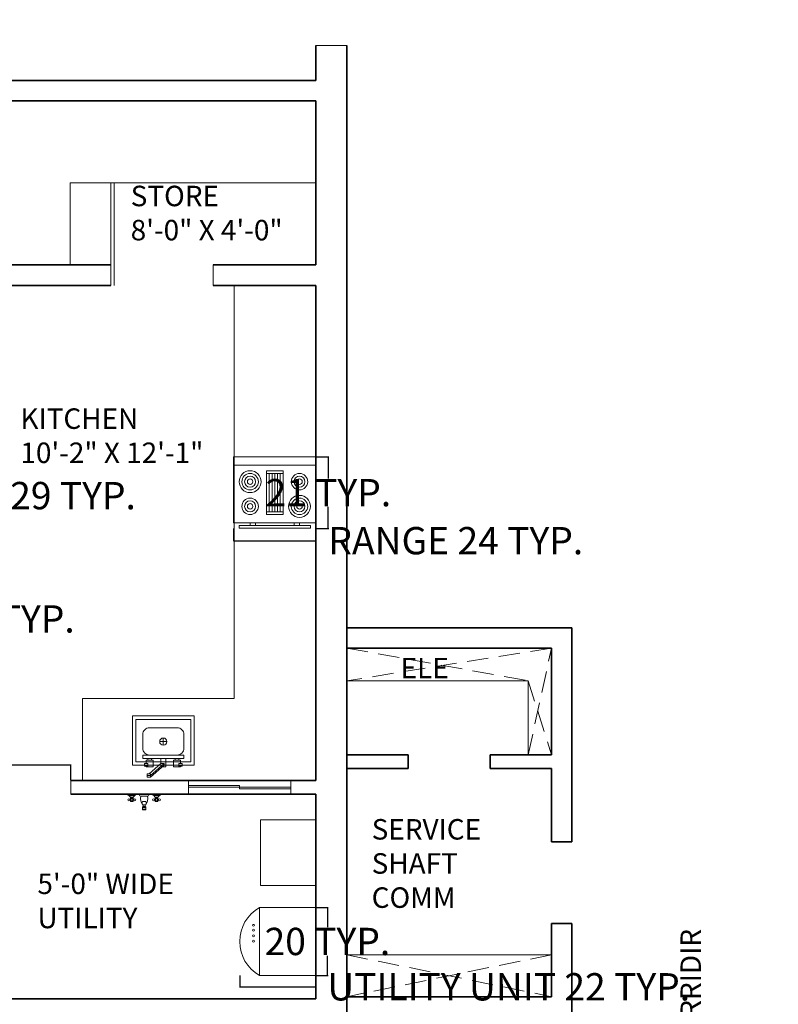
# Model space of a CAD drawing. Units: inches. Extents: x 3343 to 4790, y 1140 to 2641.
# Tile 5 of 10: x 3881 to 4104, y 2022 to 2310. Entities that reach past the tile are written whole.
import ezdxf

# ---------------------------------------------------------------- set-up
doc = ezdxf.new("R2010")
doc.units = ezdxf.units.IN
doc.header["$LTSCALE"] = 5
doc.header["$MEASUREMENT"] = 0
doc.linetypes.add('HIDDEN', pattern=[0.375, 0.25, -0.125])
for name, color, linetype, lineweight in [('A-ANNO-DIMS', 2, 'Continuous', 18), ('A-AREA-IDEN', 7, 'Continuous', 18), ('A-DOOR', 3, 'Continuous', 18), ('A-EQPM', 9, 'Continuous', 18), ('A-FLOR-CASE', 9, 'Continuous', 18), ('A-FLOR-FIXT', 9, 'Continuous', 18), ('A-FLOR-HIDN', 8, 'HIDDEN', 13), ('A-FLOR-SHFT', 8, 'Continuous', 18), ('A-GLAZ', 4, 'Continuous', 18), ('A-WALL', 7, 'Continuous', 35)]:
    doc.layers.add(name, color=color, linetype=linetype, lineweight=lineweight)
doc.styles.get("Standard").update_dxf_attribs({"font": 'arial.ttf'})
doc.dimstyles.get("Standard").update_dxf_attribs({"dimtxt": 8, "dimasz": 0.18, "dimexe": 0.18, "dimexo": 0.0625, "dimgap": 0.09, "dimtad": 0, "dimtih": 1, "dimtoh": 1, "dimdec": 1, "dimzin": 0, "dimdsep": 46, "dimlunit": 3, "dimtxsty": 'Standard', "dimcen": 0.09, "dimadec": 0, "dimazin": 0, "dimtfac": 1, "dimtdec": 1, "dimtofl": 0, "dimtmove": 0, "dimatfit": 3, "dimfxl": 1, "dimtolj": 1, "dimtzin": 0, "dimarcsym": 0})

# ---------------------------------------------------------------- blocks, each defined once
blk = doc.blocks.new('Faucet - Bathroom front')
for p, q in [((-0.5, 4.25), (0.5, 4.25)), ((0.5, 3.75), (-0.5, 3.75)), ((-0.5, 3), (0.5, 3)), ((-0.25, 3), (-0.25, 3.5)), ((0.25, 3.5), (0.25, 3)), ((-5, 0), (-2.25, 0)), ((-4.5087, 0.25), (-2.7408, 0.25)), ((-4, 1.625), (-4.25, 1.625)), ((-4, 1.375), (-4.25, 1.375)), ((-3.1442, 0.75), (-4.0979, 0.75)), ((-3.25, 1.625), (-3, 1.625)), ((-3.25, 1.375), (-3, 1.375)), ((-1.5, 0), (1.5, 0)), ((-1, 0.5), (1, 0.5)), ((0.5, 2), (-0.5, 2)), ((2.25, 0), (5, 0)), ((2.7413, 0.25), (4.5092, 0.25)), ((3.25, 1.625), (3, 1.625)), ((3.25, 1.375), (3, 1.375)), ((4.1058, 0.75), (3.1521, 0.75)), ((4, 1.625), (4.25, 1.625)), ((4, 1.375), (4.25, 1.375))]:
    blk.add_line(p, q)
for points in [[(-0.5, 3.75), (-0.5, 4.25)], [(-0.25, 4.5), (0.25, 4.5)], [(0.25, 3.5), (-0.25, 3.5)], [(0.5, 4.25), (0.5, 3.75)]]:
    blk.add_lwpolyline(points)
for points in [[(-4, 1), (-4, 2), (-3.25, 2), (-3.25, 1)], [(3.25, 1), (3.25, 2), (4, 2), (4, 1)]]:
    blk.add_lwpolyline(points, close=True)
for centre in [(-4.5, 1.5), (-3.625, 1.5), (-2.75, 1.5), (2.75, 1.5), (3.625, 1.5), (4.5, 1.5)]:
    blk.add_circle(centre, 0.2795)
for centre, radius, start, end in [((3, 1), 4.0311, 150.2551, 187.125), ((0.6413, 2.5), 1.246, 156.3417, 203.6583), ((-0.2575, 4.2575), 0.2426, 88.22243, 181.7776), ((-0.2575, 3.7425), 0.2426, 178.2224, 271.7776), ((0.2575, 4.2575), 0.2426, 358.2224, 91.77757), ((0.2575, 3.7425), 0.2426, 268.2224, 1.777565), ((-3, 1), 4.0311, 352.875, 29.74488), ((-0.6413, 2.5), 1.246, 336.3417, 23.65835), ((-5.375, 1.375), 1.4252, 285.2551, 344.7449), ((-1.875, 1.375), 1.4252, 195.2551, 254.7449), ((-0.7962, -0.2038), 0.7327, 106.1502, 163.8498), ((0.7962, -0.2038), 0.7327, 16.1502, 73.84979), ((1.875, 1.375), 1.4252, 285.2551, 344.7449), ((5.375, 1.375), 1.4252, 195.2551, 254.7449)]:
    blk.add_arc(centre, radius, start, end)
blk = doc.blocks.new('Range-Oven - 30 in top')
for p, q in [((0, -3), (30, -3)), ((12, -6), (18, -6)), ((13, -20), (13, -6)), ((14, -6), (14, -20)), ((15, -20), (15, -6)), ((16, -6), (16, -20)), ((17, -20), (17, -6)), ((18, -20), (12, -20)), ((6, -24), (6, -25)), ((8, -25), (8, -24)), ((22, -25), (22, -24)), ((24, -24), (24, -25))]:
    blk.add_line(p, q)
for points in [[(0, -24), (0, 0), (30, 0), (30, -24)], [(12, -21), (12, -5), (18, -5), (18, -21)], [(2, -26), (2, -25), (28, -25), (28, -26)]]:
    blk.add_lwpolyline(points, close=True)
for centre, radius in [((6, -9), 4), ((6, -9), 3), ((6, -9), 2), ((24, -9), 3), ((24, -9), 2), ((6, -9), 1), ((24, -9), 1), ((24, -18), 4), ((6, -18), 3), ((6, -18), 2), ((6, -18), 1), ((24, -18), 3), ((24, -18), 2), ((24, -18), 1)]:
    blk.add_circle(centre, radius)
blk = doc.blocks.new('Faucet - kit sink front')
for p, q in [((-0.25, 3), (3.75, 6.5)), ((3.75, 6), (-0.25, 2.5)), ((3.75, 6), (3.75, 6.5)), ((3.75, 6.5), (4.75, 6.5)), ((3.75, 5.5), (3.75, 6)), ((4.75, 6), (3.75, 6)), ((4.75, 6.5), (4.75, 6)), ((4.75, 6), (4.75, 5.5)), ((-0.75, 3.5), (0.3192, 3.5)), ((-0.75, 1), (-0.75, 3.5)), ((-0.25, 2.5), (-0.25, 3)), ((4.1921, 5.5041), (0.75, 2.5)), ((4.75, 5.5), (3.75, 5.5)), ((-4.5, 1), (-4.5, 1.5)), ((-3.5, 1.5), (-3.5, 1)), ((0.75, 2.5), (-0.25, 2.5)), ((0.75, 2.5), (0.75, 1)), ((3.5, 1.5), (3.5, 1)), ((4.5, 1), (4.5, 1.5))]:
    blk.add_line(p, q)
for points in [[(-5.5, 2.5), (-5.5, 3.25), (-4.5, 3.25), (-4.5, 2.5)], [(5.5, 2.5), (5.5, 3.25), (4.5, 3.25), (4.5, 2.5)], [(-6, 0), (-6, 1), (6, 1), (6, 0)]]:
    blk.add_lwpolyline(points, close=True)
for points in [[(-5, 3.2513), (-5, 3.5), (-3, 3.5), (-3, 1.5), (-5, 1.5), (-5, 2.5)], [(5, 3.2513), (5, 3.5), (3, 3.5), (3, 1.5), (5, 1.5), (5, 2.5)]]:
    blk.add_lwpolyline(points)
blk = doc.blocks.new('UTILITY-APPLIANCE')
blk.add_lwpolyline([(22.35, 19.84), (5.78, 19.84), (5.78, 0), (22.35, 0)], close=True)
for centre in [(4.05, 14.66), (4.05, 13.23), (4.05, 11.58), (4.05, 10.02)]:
    blk.add_circle(centre, 0.275)
blk.add_arc((11.41, 9.92), 11.41, 119.598, 240.402)
blk = doc.blocks.new('DOOR-30IN-4IN-JAMB-DBL-LINE')
at = {"ltscale": 5}
for p, q in [((29, 0), (29, 30)), ((30, 0), (30, 30)), ((0, 4), (0, 0)), ((30, 4), (30, 0))]:
    blk.add_line(p, q, dxfattribs=at)
blk = doc.blocks.new('*D51')
at = {"layer": 'A-ANNO-DIMS', "color": 0, "lineweight": -2, "ltscale": 5, "transparency": 16777216}
for p, q in [((3806.15, 2137.1), (3806.15, 2134.27)), ((3824.22, 2137.1), (3824.22, 2134.27)), ((3806.33, 2134.45), (3824.04, 2134.45)), ((3824.22, 2134.45), (3824.4, 2134.45))]:
    blk.add_line(p, q, dxfattribs=at)
at = {"layer": 'A-ANNO-DIMS', "color": 0, "ltscale": 5, "transparency": 16777216}
for points in [[(3806.33, 2134.48), (3806.33, 2134.42), (3806.15, 2134.45)], [(3824.04, 2134.48), (3824.04, 2134.42), (3824.22, 2134.45)]]:
    blk.add_solid(points, dxfattribs=at)
at = {"layer": 'Defpoints', "color": 0, "ltscale": 5, "transparency": 16777216}
for p in [(3806.15, 2137.16), (3824.22, 2137.16), (3824.22, 2134.45)]:
    blk.add_point(p, dxfattribs=at)
at = {"layer": 'A-ANNO-DIMS', "color": 0, "ltscale": 5, "transparency": 16777216, "insert": (3862.1, 2134.45), "char_height": 8, "attachment_point": 5}
blk.add_mtext('\\A1;BASIN 18 TYP.', dxfattribs=at)
blk = doc.blocks.new('*D69')
at = {"layer": 'A-ANNO-DIMS', "color": 0, "lineweight": -2, "ltscale": 5, "transparency": 16777216}
for p, q in [((3944.01, 2160.92), (3944.01, 2157.19)), ((3968.13, 2160.92), (3968.13, 2157.19)), ((3944.19, 2157.37), (3967.95, 2157.37)), ((3968.13, 2157.37), (3968.31, 2157.37))]:
    blk.add_line(p, q, dxfattribs=at)
at = {"layer": 'A-ANNO-DIMS', "color": 0, "ltscale": 5, "transparency": 16777216}
for points in [[(3944.19, 2157.4), (3944.19, 2157.34), (3944.01, 2157.37)], [(3967.95, 2157.4), (3967.95, 2157.34), (3968.13, 2157.37)]]:
    blk.add_solid(points, dxfattribs=at)
at = {"layer": 'Defpoints', "color": 0, "ltscale": 5, "transparency": 16777216}
for p in [(3944.01, 2160.98), (3968.13, 2160.98), (3968.13, 2157.37)]:
    blk.add_point(p, dxfattribs=at)
at = {"layer": 'A-ANNO-DIMS', "color": 0, "ltscale": 5, "transparency": 16777216, "insert": (4009.09, 2157.37), "char_height": 8, "attachment_point": 5}
blk.add_mtext('\\A1;RANGE 24 TYP.', dxfattribs=at)
blk = doc.blocks.new('*D70')
at = {"layer": 'A-ANNO-DIMS', "color": 0, "lineweight": -2, "ltscale": 5, "transparency": 16777216}
for p, q in [((3968.19, 2181.88), (3971.93, 2181.88)), ((3971.75, 2181.7), (3971.75, 2175.54)), ((3971.75, 2161.16), (3971.75, 2167.32)), ((3968.19, 2160.98), (3971.93, 2160.98))]:
    blk.add_line(p, q, dxfattribs=at)
at = {"layer": 'A-ANNO-DIMS', "color": 0, "ltscale": 5, "transparency": 16777216}
for points in [[(3971.72, 2181.7), (3971.78, 2181.7), (3971.75, 2181.88)], [(3971.72, 2161.16), (3971.78, 2161.16), (3971.75, 2160.98)]]:
    blk.add_solid(points, dxfattribs=at)
at = {"layer": 'Defpoints', "color": 0, "ltscale": 5, "transparency": 16777216}
for p in [(3968.13, 2181.88), (3971.75, 2181.88), (3968.13, 2160.98)]:
    blk.add_point(p, dxfattribs=at)
at = {"layer": 'A-ANNO-DIMS', "color": 0, "ltscale": 5, "transparency": 16777216, "insert": (3971.75, 2171.43), "char_height": 8, "attachment_point": 5}
blk.add_mtext('\\A1;21 TYP.', dxfattribs=at)
blk = doc.blocks.new('*D72')
at = {"layer": 'A-ANNO-DIMS', "color": 0, "lineweight": -2, "ltscale": 5, "transparency": 16777216}
for p, q in [((3848.13, 2165.23), (3848.13, 2170.75)), ((3848.31, 2170.57), (3876.95, 2170.57)), ((3877.13, 2165.23), (3877.13, 2170.75)), ((3877.13, 2170.57), (3877.31, 2170.57))]:
    blk.add_line(p, q, dxfattribs=at)
at = {"layer": 'A-ANNO-DIMS', "color": 0, "ltscale": 5, "transparency": 16777216}
for points in [[(3848.31, 2170.6), (3848.31, 2170.54), (3848.13, 2170.57)], [(3876.95, 2170.6), (3876.95, 2170.54), (3877.13, 2170.57)]]:
    blk.add_solid(points, dxfattribs=at)
at = {"layer": 'Defpoints', "color": 0, "ltscale": 5, "transparency": 16777216}
for p in [(3877.13, 2170.57), (3848.13, 2165.17), (3877.13, 2165.17)]:
    blk.add_point(p, dxfattribs=at)
at = {"layer": 'A-ANNO-DIMS', "color": 0, "ltscale": 5, "transparency": 16777216, "insert": (3896.94, 2170.57), "char_height": 8, "attachment_point": 5}
blk.add_mtext('\\A1;29 TYP.', dxfattribs=at)
blk = doc.blocks.new('*D73')
at = {"layer": 'A-ANNO-DIMS', "color": 0, "lineweight": -2, "ltscale": 5, "transparency": 16777216}
for p, q in [((3945.78, 2029.98), (3945.78, 2026.51)), ((3968.13, 2029.98), (3968.13, 2026.51)), ((3945.96, 2026.69), (3967.95, 2026.69)), ((3968.13, 2026.69), (3968.31, 2026.69))]:
    blk.add_line(p, q, dxfattribs=at)
at = {"layer": 'A-ANNO-DIMS', "color": 0, "ltscale": 5, "transparency": 16777216}
for points in [[(3945.96, 2026.72), (3945.96, 2026.66), (3945.78, 2026.69)], [(3967.95, 2026.72), (3967.95, 2026.66), (3968.13, 2026.69)]]:
    blk.add_solid(points, dxfattribs=at)
at = {"layer": 'Defpoints', "color": 0, "ltscale": 5, "transparency": 16777216}
for p in [(3945.78, 2030.05), (3968.13, 2030.05), (3968.13, 2026.69)]:
    blk.add_point(p, dxfattribs=at)
at = {"layer": 'A-ANNO-DIMS', "color": 0, "ltscale": 5, "transparency": 16777216, "insert": (4024.61, 2026.69), "char_height": 8, "attachment_point": 5}
blk.add_mtext('\\A1;UTILITY UNIT 22 TYP.', dxfattribs=at)
blk = doc.blocks.new('*D74')
at = {"layer": 'A-ANNO-DIMS', "color": 0, "lineweight": -2, "ltscale": 5, "transparency": 16777216}
for p, q in [((3968.19, 2049.89), (3971.66, 2049.89)), ((3971.48, 2049.71), (3971.48, 2044.14)), ((3971.48, 2030.23), (3971.48, 2035.79)), ((3968.19, 2030.05), (3971.66, 2030.05))]:
    blk.add_line(p, q, dxfattribs=at)
at = {"layer": 'A-ANNO-DIMS', "color": 0, "ltscale": 5, "transparency": 16777216}
for points in [[(3971.45, 2049.71), (3971.51, 2049.71), (3971.48, 2049.89)], [(3971.45, 2030.23), (3971.51, 2030.23), (3971.48, 2030.05)]]:
    blk.add_solid(points, dxfattribs=at)
at = {"layer": 'Defpoints', "color": 0, "ltscale": 5, "transparency": 16777216}
for p in [(3968.13, 2049.89), (3971.48, 2049.89), (3968.13, 2030.05)]:
    blk.add_point(p, dxfattribs=at)
at = {"layer": 'A-ANNO-DIMS', "color": 0, "ltscale": 5, "transparency": 16777216, "insert": (3971.48, 2039.97), "char_height": 8, "attachment_point": 5}
blk.add_mtext('\\A1;20 TYP.', dxfattribs=at)
blk = doc.blocks.new('*D81')
at = {"layer": 'A-ANNO-DIMS', "color": 0, "lineweight": -2, "ltscale": 5, "transparency": 16777216}
for p, q in [((3866.27, 2091.66), (3866.09, 2091.66)), ((3866.27, 2087.22), (3866.27, 2091.84)), ((3896.09, 2091.66), (3866.45, 2091.66)), ((3896.27, 2087.22), (3896.27, 2091.84))]:
    blk.add_line(p, q, dxfattribs=at)
at = {"layer": 'A-ANNO-DIMS', "color": 0, "ltscale": 5, "transparency": 16777216}
for points in [[(3866.45, 2091.69), (3866.45, 2091.63), (3866.27, 2091.66)], [(3896.09, 2091.69), (3896.09, 2091.63), (3896.27, 2091.66)]]:
    blk.add_solid(points, dxfattribs=at)
at = {"layer": 'Defpoints', "color": 0, "ltscale": 5, "transparency": 16777216}
for p in [(3866.27, 2091.66), (3866.27, 2087.16), (3896.27, 2087.16)]:
    blk.add_point(p, dxfattribs=at)
at = {"layer": 'A-ANNO-DIMS', "color": 0, "ltscale": 5, "transparency": 16777216, "insert": (3828.41, 2091.66), "char_height": 8, "attachment_point": 5}
blk.add_mtext('\\A1;DOOR 30 TYP.', dxfattribs=at)
blk = doc.blocks.new('*D83')
at = {"layer": 'A-ANNO-DIMS', "color": 0, "lineweight": -2, "ltscale": 5, "transparency": 16777216}
for p, q in [((3424.13, 2432.05), (3424.13, 2635.49)), ((3424.31, 2635.31), (4052.48, 2635.31)), ((4703.95, 2635.31), (4075.77, 2635.31)), ((4704.13, 2197.22), (4704.13, 2635.49))]:
    blk.add_line(p, q, dxfattribs=at)
at = {"layer": 'A-ANNO-DIMS', "color": 0, "ltscale": 5, "transparency": 16777216}
for points in [[(3424.31, 2635.34), (3424.31, 2635.28), (3424.13, 2635.31)], [(4703.95, 2635.34), (4703.95, 2635.28), (4704.13, 2635.31)]]:
    blk.add_solid(points, dxfattribs=at)
at = {"layer": 'Defpoints', "color": 0, "ltscale": 5, "transparency": 16777216}
for p in [(4704.13, 2635.31), (3424.13, 2431.99), (4704.13, 2197.16)]:
    blk.add_point(p, dxfattribs=at)
at = {"layer": 'A-ANNO-DIMS', "color": 0, "ltscale": 5, "transparency": 16777216, "insert": (4064.13, 2635.31), "char_height": 8, "attachment_point": 5}
blk.add_mtext('\\A1;1280', dxfattribs=at)
blk = doc.blocks.new('*D84')
at = {"layer": 'A-ANNO-DIMS', "color": 0, "lineweight": -2, "ltscale": 5, "transparency": 16777216}
for p, q in [((3448.07, 2566.16), (3354.8, 2566.16)), ((3354.98, 2565.98), (3354.98, 1894.31)), ((3354.98, 1214.29), (3354.98, 1885.96)), ((4015.58, 1214.11), (3354.8, 1214.11))]:
    blk.add_line(p, q, dxfattribs=at)
at = {"layer": 'A-ANNO-DIMS', "color": 0, "ltscale": 5, "transparency": 16777216}
for points in [[(3354.95, 2565.98), (3355.01, 2565.98), (3354.98, 2566.16)], [(3354.95, 1214.29), (3355.01, 1214.29), (3354.98, 1214.11)]]:
    blk.add_solid(points, dxfattribs=at)
at = {"layer": 'Defpoints', "color": 0, "ltscale": 5, "transparency": 16777216}
for p in [(3448.13, 2566.16), (3354.98, 1214.11), (4015.65, 1214.11)]:
    blk.add_point(p, dxfattribs=at)
at = {"layer": 'A-ANNO-DIMS', "color": 0, "ltscale": 5, "transparency": 16777216, "insert": (3354.98, 1890.14), "char_height": 8, "attachment_point": 5}
blk.add_mtext('\\A1;1352', dxfattribs=at)
blk = doc.blocks.new('*D87')
at = {"layer": 'A-ANNO-DIMS', "color": 0, "lineweight": -2, "ltscale": 5, "transparency": 16777216}
for p, q in [((3977.19, 2566.16), (4773.46, 2566.16)), ((4773.28, 2565.98), (4773.28, 2294.34)), ((4773.28, 2014.34), (4773.28, 2285.99)), ((3977.19, 2014.16), (4773.46, 2014.16))]:
    blk.add_line(p, q, dxfattribs=at)
at = {"layer": 'A-ANNO-DIMS', "color": 0, "ltscale": 5, "transparency": 16777216}
for points in [[(4773.25, 2565.98), (4773.31, 2565.98), (4773.28, 2566.16)], [(4773.25, 2014.34), (4773.31, 2014.34), (4773.28, 2014.16)]]:
    blk.add_solid(points, dxfattribs=at)
at = {"layer": 'Defpoints', "color": 0, "ltscale": 5, "transparency": 16777216}
for p in [(3977.13, 2566.16), (3977.13, 2014.16), (4773.28, 2014.16)]:
    blk.add_point(p, dxfattribs=at)
at = {"layer": 'A-ANNO-DIMS', "color": 0, "ltscale": 5, "transparency": 16777216, "insert": (4773.28, 2290.16), "char_height": 8, "attachment_point": 5}
blk.add_mtext('\\A1;552', dxfattribs=at)

msp = doc.modelspace()

# ---------------------------------------------------------------- linework, layer by layer
at = {"layer": 'A-DOOR', "ltscale": 5}
for p, q in [((3977.13, 2302.46), (3968.13, 2302.46)), ((3907.995, 2232.161), (3907.995, 2262.161)), ((3908.995, 2232.161), (3908.995, 2262.161)), ((3907.995, 2238.161), (3907.995, 2232.161)), ((3937.995, 2238.161), (3937.995, 2232.161))]:
    msp.add_line(p, q, dxfattribs=at)
at = {"layer": 'A-EQPM'}
msp.add_lwpolyline([(3968.13, 2075.551), (3951.908, 2075.551), (3951.908, 2056.328), (3968.13, 2056.328)], close=True, dxfattribs=at)
at = {"layer": 'A-FLOR-CASE'}
for p, q in [((3896.13, 2262.161), (3896.13, 2238.161)), ((3944.13, 2232.161), (3944.13, 2111.161))]:
    msp.add_line(p, q, dxfattribs=at)
at = {"layer": 'A-FLOR-CASE', "ltscale": 5}
for p, q in [((3968.13, 2262.161), (3896.13, 2262.161)), ((3944.13, 2111.161), (3899.684, 2111.161)), ((3899.684, 2087.161), (3899.684, 2111.161))]:
    msp.add_line(p, q, dxfattribs=at)
at = {"layer": 'A-FLOR-FIXT'}
for p, q in [((3924.467, 2098.496), (3922.348, 2098.496)), ((3923.407, 2097.436), (3923.407, 2099.556))]:
    msp.add_line(p, q, dxfattribs=at)
for points in [[(3914.376, 2091.584), (3914.376, 2106.021), (3932.439, 2106.021), (3932.439, 2091.584)], [(3915.376, 2105.021), (3931.439, 2105.021), (3931.439, 2092.584), (3915.376, 2092.584)]]:
    msp.add_lwpolyline(points, close=True, dxfattribs=at)
msp.add_lwpolyline([(3929.439, 2096.584), (3929.439, 2100.584, 0.4142136), (3927.439, 2102.584), (3919.376, 2102.584, 0.4142136), (3917.376, 2100.584), (3917.376, 2096.584, 0.4142136), (3919.376, 2094.584), (3927.439, 2094.584, 0.4142136)], format="xyb", close=True, dxfattribs=at)
msp.add_circle((3923.407, 2098.496), 1.06, dxfattribs=at)
at = {"layer": 'A-FLOR-HIDN', "ltscale": 5}
for p, q in [((3977.13, 2125.871), (4030.31, 2116.333)), ((4037.13, 2125.871), (3977.13, 2116.333)), ((4030.31, 2094.599), (4037.13, 2125.871)), ((4030.31, 2116.333), (4037.13, 2094.599)), ((4037.13, 2036.063), (3977.13, 2023.79)), ((3977.13, 2036.063), (4037.13, 2023.79))]:
    msp.add_line(p, q, dxfattribs=at)
at = {"layer": 'A-FLOR-SHFT', "ltscale": 5}
for p, q in [((3977.13, 2116.333), (4030.31, 2116.333)), ((4030.31, 2116.333), (4030.31, 2094.599)), ((3977.13, 2036.063), (4037.13, 2036.063))]:
    msp.add_line(p, q, dxfattribs=at)
at = {"layer": 'A-GLAZ', "ltscale": 5}
for p, q in [((3930.773, 2087.161), (3930.773, 2083.161)), ((3930.773, 2085.661), (3945.773, 2085.661)), ((3945.773, 2085.661), (3945.773, 2084.661)), ((3960.773, 2087.161), (3960.773, 2083.161)), ((3930.773, 2085.161), (3960.773, 2085.161)), ((3945.773, 2084.661), (3960.773, 2084.661))]:
    msp.add_line(p, q, dxfattribs=at)
at = {"layer": 'A-WALL'}
for p, q in [((3968.13, 2302.46), (3968.13, 2292.161)), ((3977.13, 2302.46), (3977.13, 2014.161)), ((3968.13, 2286.161), (3968.13, 2238.161)), ((3968.13, 2232.161), (3968.13, 2087.161)), ((4043.13, 2131.871), (4043.13, 2069.194)), ((4037.13, 2125.871), (4037.13, 2094.599)), ((4037.13, 2090.599), (4037.13, 2069.194)), ((3968.13, 2083.161), (3968.13, 2023.161)), ((4037.13, 2045.194), (4037.13, 2023.79)), ((4043.13, 2045.194), (4043.13, 2002.915))]:
    msp.add_line(p, q, dxfattribs=at)
at = {"layer": 'A-WALL', "ltscale": 5}
for p, q in [((3894.654, 2292.161), (3818.13, 2292.161)), ((3968.13, 2292.161), (3894.654, 2292.161)), ((3894.654, 2286.161), (3872.13, 2286.161)), ((3968.13, 2286.161), (3894.654, 2286.161)), ((3907.995, 2238.161), (3872.13, 2238.161)), ((3968.13, 2238.161), (3937.995, 2238.161)), ((3907.995, 2232.161), (3818.13, 2232.161)), ((3968.13, 2232.161), (3937.995, 2232.161)), ((4043.13, 2131.871), (3977.13, 2131.871)), ((4037.13, 2125.871), (3977.13, 2125.871)), ((3977.13, 2094.599), (3995.13, 2094.599)), ((3995.13, 2090.599), (3995.13, 2094.599)), ((4019.13, 2090.599), (4019.13, 2094.599)), ((4019.13, 2094.599), (4037.13, 2094.599)), ((3977.13, 2090.599), (3995.13, 2090.599)), ((4019.13, 2090.599), (4037.13, 2090.599)), ((3968.13, 2087.161), (3896.266, 2087.161)), ((3968.13, 2083.161), (3896.266, 2083.161)), ((4037.13, 2069.194), (4043.13, 2069.194)), ((4037.13, 2045.194), (4043.13, 2045.194)), ((3968.13, 2023.161), (3848.13, 2023.161)), ((3977.13, 2023.79), (4037.13, 2023.79))]:
    msp.add_line(p, q, dxfattribs=at)

# ---------------------------------------------------------------- block references
at = {"layer": 'A-DOOR', "rotation": 180}
msp.add_blockref('DOOR-30IN-4IN-JAMB-DBL-LINE', (3896.266, 2087.161), dxfattribs=at)
at = {"layer": 'A-EQPM', "xscale": 0.8038317938248679, "yscale": 0.8038317938248679, "zscale": 0.8038317938248679}
msp.add_blockref('Range-Oven - 30 in top', (3944.015, 2181.883), dxfattribs=at)
at = {"layer": 'A-EQPM'}
msp.add_blockref('UTILITY-APPLIANCE', (3945.775, 2030.048), dxfattribs=at)
at = {"layer": 'A-FLOR-FIXT', "rotation": 180}
for name, p in [('Faucet - kit sink front', (3923.407, 2094.584)), ('Faucet - Bathroom front', (3917.795, 2082.983))]:
    msp.add_blockref(name, p, dxfattribs=at)

# ---------------------------------------------------------------- texts
at = {"layer": 'A-AREA-IDEN', "ltscale": 5, "char_height": 6, "attachment_point": 1}
for s, insert in [('STORE\\P8\'-0" X 4\'-0"', (3913.845, 2261.334)), ('KITCHEN\\P10\'-2" X 12\'-1"', (3881.539, 2196.118)), ('ELE', (3992.943, 2123.035)), ('SERVICE\\PSHAFT\\PCOMM', (3984.454, 2075.822)), ('5\'-0" WIDE \\PUTILITY', (3886.523, 2059.859))]:
    msp.add_mtext_dynamic_manual_height_columns(s, width=189.69543, gutter_width=1, heights=[0], dxfattribs=dict(at, insert=insert))
at = {"layer": 'A-AREA-IDEN', "ltscale": 5, "insert": (4074.933, 1964.53), "char_height": 6, "attachment_point": 1, "rotation": 90}
msp.add_mtext_dynamic_manual_height_columns('6\'-6" WIDE CORRIDIR', width=189.69543, gutter_width=1, heights=[0], dxfattribs=at)

# ---------------------------------------------------------------- dimensions: what is measured, and where the dimension line sits
at = {"layer": 'A-ANNO-DIMS', "ltscale": 5}
dim = msp.add_linear_dim(base=(4704.13, 2635.311), p1=(3424.13, 2431.992), p2=(4704.13, 2197.161), dimstyle='Standard', override={"dimdec": 0, "dimlfac": 1, "dimrnd": 0, "dimzin": 0, "dimdsep": 46, "dimlunit": 2}, dxfattribs=at)
dim.commit()
dim.dimension.update_dxf_attribs({"geometry": '*D83', "text_midpoint": (4064.13, 2635.311)})
for base, p1, p2, picture, middle in [((3354.98, 1214.112), (3448.13, 2566.161), (4015.647, 1214.112), '*D84', (3354.98, 1890.137)), ((4773.28, 2014.161), (3977.13, 2566.161), (3977.13, 2014.161), '*D87', (4773.28, 2290.161))]:
    dim = msp.add_linear_dim(base=base, p1=p1, p2=p2, angle=90, dimstyle='Standard', override={"dimdec": 0, "dimlfac": 1, "dimrnd": 0, "dimzin": 0, "dimdsep": 46, "dimlunit": 2}, dxfattribs=at)
    dim.commit()
    dim.dimension.update_dxf_attribs({"geometry": picture, "text_midpoint": middle})
for base, p1, p2, angle, text, picture, middle in [((3971.747, 2181.883), (3968.13, 2160.983), (3968.13, 2181.883), 90, '<> TYP.', '*D70', (3971.747, 2171.433)), ((3866.266, 2091.661), (3896.266, 2087.161), (3866.266, 2087.161), 180, 'DOOR <> TYP.', '*D81', (3828.408, 2091.661)), ((3971.483, 2049.892), (3968.13, 2030.047), (3968.13, 2049.892), 90, '<> TYP.', '*D74', (3971.483, 2039.969))]:
    dim = msp.add_linear_dim(base=base, p1=p1, p2=p2, angle=angle, text=text, dimstyle='Standard', override={"dimdec": 0, "dimlfac": 1, "dimrnd": 0, "dimzin": 0, "dimdsep": 46, "dimlunit": 2}, dxfattribs=at)
    dim.commit()
    dim.dimension.update_dxf_attribs({"geometry": picture, "text_midpoint": middle})
for base, p1, p2, text, picture, middle in [((3877.13, 2170.566), (3848.13, 2165.166), (3877.13, 2165.166), '<> TYP.', '*D72', (3896.938, 2170.566)), ((3968.13, 2157.366), (3944.015, 2160.983), (3968.13, 2160.983), 'RANGE <> TYP.', '*D69', (4009.087, 2157.366)), ((3824.217, 2134.452), (3806.155, 2137.161), (3824.217, 2137.161), 'BASIN <> TYP.', '*D51', (3862.102, 2134.452)), ((3968.13, 2026.694), (3945.775, 2030.047), (3968.13, 2030.047), 'UTILITY UNIT <> TYP.', '*D73', (4024.607, 2026.694))]:
    dim = msp.add_linear_dim(base=base, p1=p1, p2=p2, text=text, dimstyle='Standard', override={"dimdec": 0, "dimlfac": 1, "dimrnd": 0, "dimzin": 0, "dimdsep": 46, "dimlunit": 2}, dxfattribs=at)
    dim.commit()
    dim.dimension.update_dxf_attribs({"geometry": picture, "text_midpoint": middle})

doc.saveas('drawing.dxf')
